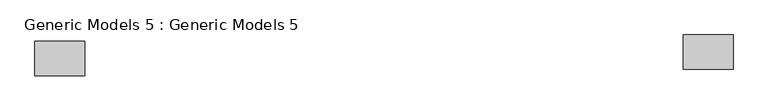
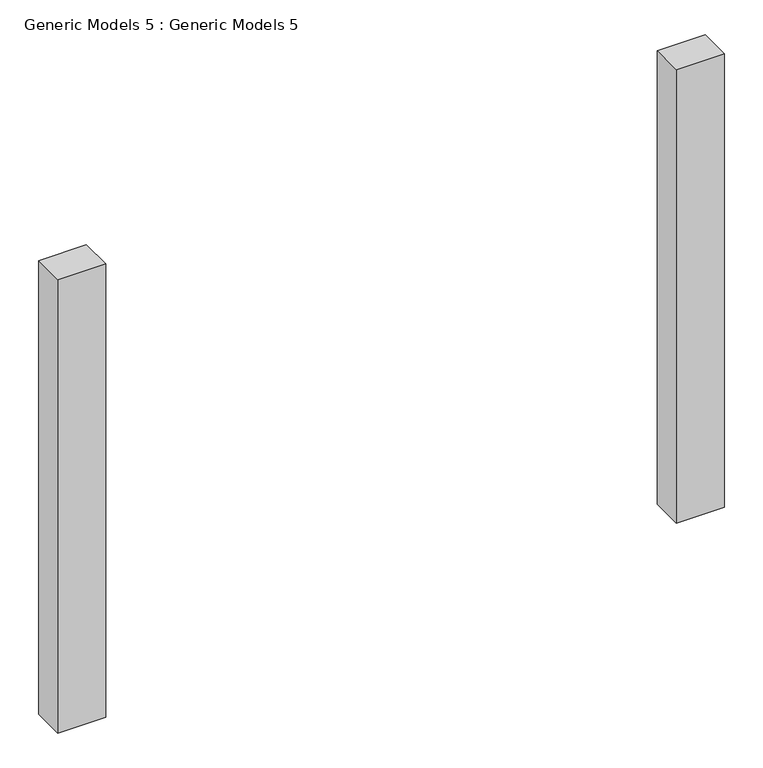
"""IFC4 building model written with IfcOpenShell, lengths in millimetres: proxy geometry, Generic Models 5 : Generic Models 5."""

from ifc_helpers import new_model, si_unit, frame, origin, place, context, project, spatial, polyline, outline, extrude, source, transform, mapped, element, save


def generic_models_5_generic_models_5_3b624c68(model_context):
    return source(origin(), model_context, "Body", "SweptSolid", [
        extrude(outline(polyline([(-3160.3486505, -6994.3736114), (-3312.7486505, -6994.3736114), (-3312.7486505, -6889.3546951), (-3160.3486505, -6889.3546951), (-3160.3486505, -6994.3736114)])), frame((0.0, 0.0, -457.2), z_axis=(0.0, 0.0, 1.0), x_axis=(1.0, 0.0, 0.0)), (0.0, 0.0, 1.0), 1524.0),
        extrude(outline(polyline([(-1181.0544048, -6974.4930164), (-1333.4544048, -6974.4930164), (-1333.4544048, -6869.4741001), (-1181.0544048, -6869.4741001), (-1181.0544048, -6974.4930164)])), frame((0.0, 0.0, -457.2), z_axis=(0.0, 0.0, 1.0), x_axis=(1.0, 0.0, 0.0)), (0.0, 0.0, 1.0), 1524.0),
    ])


if __name__ == "__main__":
    model = new_model("IFC4")
    model_context = context("Model", 3, world=origin())
    ifc_project = project(units=[si_unit("LENGTHUNIT", "METRE", prefix="MILLI")], contexts=[model_context])
    site = spatial("IfcSite", under=ifc_project)
    building = spatial("IfcBuilding", under=site)
    placement = place(None, origin())
    generic_models_5_generic_models_5_shape = generic_models_5_generic_models_5_3b624c68(model_context)
    element("IfcBuildingElementProxy", 1, Name="Generic Models 5 : Generic Models 5", ObjectType="Generic Models 5 : Generic Models 5", at=placement, inside=building, context=model_context, shape_type="MappedRepresentation", body=[
        mapped(generic_models_5_generic_models_5_shape, transform((0.0, 0.0, 0.0), x_axis=(1.0, 0.0, 0.0), y_axis=(0.0, 1.0, 0.0), z_axis=(0.0, 0.0, 1.0))),
    ])
    save(model, "model.ifc")
